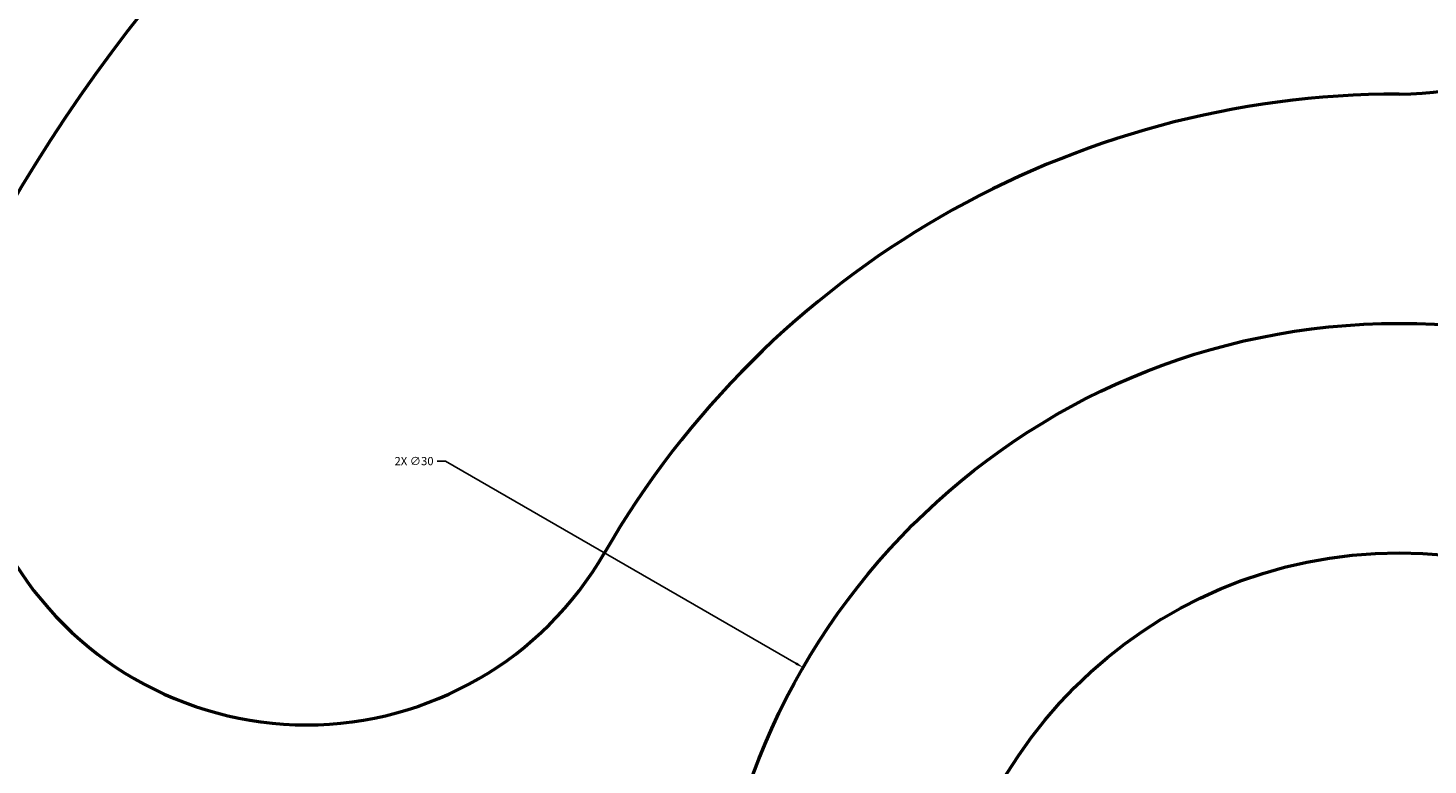
# Model space of a CAD drawing. Units: inches. Extents: x 413 to 622, y 326 to 447.
# Tile 4 of 15: x 443 to 473, y 392 to 408. Entities that reach past the tile are written whole.
import ezdxf

# ---------------------------------------------------------------- set-up
doc = ezdxf.new("R2010")
doc.units = ezdxf.units.IN
doc.header["$MEASUREMENT"] = 0
doc.layers.add('M-DIMS', color=2, linetype='Continuous', lineweight=18)
doc.layers.add('M-OUTL', color=7, linetype='Continuous', lineweight=50)
doc.styles.get("Standard").update_dxf_attribs({"font": 'arial.ttf'})
doc.dimstyles.get("Standard").update_dxf_attribs({"dimtxt": 0.18, "dimasz": 0.18, "dimexe": 0.18, "dimexo": 0.0625, "dimgap": 0.09, "dimtad": 0, "dimtih": 1, "dimtoh": 1, "dimdec": 4, "dimzin": 0, "dimdsep": 46, "dimtxsty": 'Standard', "dimcen": 0.09, "dimadec": 0, "dimazin": 0, "dimtfac": 1, "dimtdec": 4, "dimtofl": 0, "dimtmove": 0, "dimatfit": 3, "dimfxl": 1, "dimtolj": 1, "dimtzin": 0, "dimarcsym": 0})

# ---------------------------------------------------------------- blocks, each defined once
blk = doc.blocks.new('SPROCKET-HUB-BORE')
for radius in [15, 10]:
    blk.add_circle((15, 15), radius)
blk = doc.blocks.new('SPROCKET-WEB-SLOT')
for centre, radius, start, end in [((7.501, 21.25), 7.5, 30, 210), ((31.317, 35), 20, 210, 270), ((31.317, 35), 35, 210, 270), ((31.317, 7.5), 7.5, 270, 90)]:
    blk.add_arc(centre, radius, start, end)
blk = doc.blocks.new('*D10')
at = {"layer": 'Defpoints', "color": 0, "transparency": 16777216}
for p in [(413.283, 436.392), (472.684, 436.392), (472.684, 336.392)]:
    blk.add_point(p, dxfattribs=at)
at = {"layer": 'M-DIMS', "color": 0, "lineweight": -2, "transparency": 16777216}
for p, q in [((472.621, 436.392), (413.103, 436.392)), ((413.283, 436.212), (413.283, 386.573)), ((413.283, 336.572), (413.283, 386.21)), ((472.621, 336.392), (413.103, 336.392))]:
    blk.add_line(p, q, dxfattribs=at)
at = {"layer": 'M-DIMS', "color": 0, "transparency": 16777216}
for points in [[(413.253, 436.212), (413.313, 436.212), (413.283, 436.392)], [(413.253, 336.572), (413.313, 336.572), (413.283, 336.392)]]:
    blk.add_solid(points, dxfattribs=at)
at = {"layer": 'M-DIMS', "color": 0, "transparency": 16777216, "insert": (413.283, 386.392), "char_height": 0.18, "attachment_point": 5}
blk.add_mtext('\\A1;100', dxfattribs=at)
blk = doc.blocks.new('*D11')
at = {"layer": 'Defpoints', "color": 0, "transparency": 16777216}
for p in [(621.66, 446.422), (621.66, 388.074), (423.314, 378.888)]:
    blk.add_point(p, dxfattribs=at)
at = {"layer": 'M-DIMS', "color": 0, "lineweight": -2, "transparency": 16777216}
for p, q in [((423.314, 378.95), (423.314, 446.602)), ((621.66, 388.137), (621.66, 446.602)), ((423.494, 446.422), (522.031, 446.422)), ((621.48, 446.422), (522.943, 446.422))]:
    blk.add_line(p, q, dxfattribs=at)
at = {"layer": 'M-DIMS', "color": 0, "transparency": 16777216}
for points in [[(423.494, 446.452), (423.494, 446.392), (423.314, 446.422)], [(621.48, 446.452), (621.48, 446.392), (621.66, 446.422)]]:
    blk.add_solid(points, dxfattribs=at)
at = {"layer": 'M-DIMS', "color": 0, "transparency": 16777216, "insert": (522.487, 446.422), "char_height": 0.18, "attachment_point": 5}
blk.add_mtext('\\A1;198.35', dxfattribs=at)
blk = doc.blocks.new('*D13')
at = {"layer": 'Defpoints', "color": 0, "transparency": 16777216}
for p in [(413.283, 431.392), (472.684, 431.392), (472.684, 386.392)]:
    blk.add_point(p, dxfattribs=at)
at = {"layer": 'M-DIMS', "color": 0, "lineweight": -2, "transparency": 16777216}
for p, q in [((472.621, 431.392), (413.103, 431.392)), ((413.283, 431.212), (413.283, 409.073)), ((413.283, 386.572), (413.283, 408.71)), ((472.621, 386.392), (413.103, 386.392))]:
    blk.add_line(p, q, dxfattribs=at)
at = {"layer": 'M-DIMS', "color": 0, "transparency": 16777216}
for points in [[(413.253, 431.212), (413.313, 431.212), (413.283, 431.392)], [(413.253, 386.572), (413.313, 386.572), (413.283, 386.392)]]:
    blk.add_solid(points, dxfattribs=at)
at = {"layer": 'M-DIMS', "color": 0, "transparency": 16777216, "insert": (413.283, 408.892), "char_height": 0.18, "attachment_point": 5}
blk.add_mtext('\\A1;45', dxfattribs=at)
blk = doc.blocks.new('*D26')
at = {"layer": 'Defpoints', "color": 0, "transparency": 16777216}
for p in [(459.693, 393.89), (485.675, 378.893)]:
    blk.add_point(p, dxfattribs=at)
at = {"layer": 'M-DIMS', "color": 0, "lineweight": -2, "transparency": 16777216}
for p, q in [((451.718, 398.39), (451.898, 398.39)), ((451.898, 398.39), (459.537, 393.98)), ((472.594, 386.392), (472.774, 386.392)), ((472.684, 386.302), (472.684, 386.482))]:
    blk.add_line(p, q, dxfattribs=at)
at = {"layer": 'M-DIMS', "color": 0, "transparency": 16777216}
blk.add_solid([(459.552, 394.006), (459.522, 393.954), (459.693, 393.89)], dxfattribs=at)
at = {"layer": 'M-DIMS', "color": 0, "transparency": 16777216, "insert": (451.211, 398.39), "char_height": 0.18, "attachment_point": 5}
blk.add_mtext('\\A1;2X ∅30', dxfattribs=at)
blk = doc.blocks.new('*D28')
at = {"layer": 'Defpoints', "color": 0, "transparency": 16777216}
for p in [(455.184, 416.702), (472.684, 386.392)]:
    blk.add_point(p, dxfattribs=at)
at = {"layer": 'M-DIMS', "color": 0, "lineweight": -2, "transparency": 16777216}
for p, q in [((444.504, 434.889), (444.684, 434.889)), ((444.684, 434.889), (455.094, 416.858)), ((472.594, 386.392), (472.774, 386.392)), ((472.684, 386.302), (472.684, 386.482))]:
    blk.add_line(p, q, dxfattribs=at)
at = {"layer": 'M-DIMS', "color": 0, "transparency": 16777216}
blk.add_solid([(455.12, 416.873), (455.068, 416.843), (455.184, 416.702)], dxfattribs=at)
at = {"layer": 'M-DIMS', "color": 0, "transparency": 16777216, "insert": (444.005, 434.889), "char_height": 0.18, "attachment_point": 5}
blk.add_mtext('\\A1;3X R35', dxfattribs=at)

msp = doc.modelspace()

# ---------------------------------------------------------------- linework, layer by layer
at = {"layer": 'M-OUTL'}
msp.add_circle((472.6836, 386.3915), 40, dxfattribs=at)

# ---------------------------------------------------------------- block references
at = {"layer": 'M-OUTL', "rotation": 239.9999999999996}
msp.add_blockref('SPROCKET-WEB-SLOT', (458.0314, 431.0122), dxfattribs=at)
at = {"layer": 'M-OUTL'}
msp.add_blockref('SPROCKET-HUB-BORE', (457.684, 371.392), dxfattribs=at)

# ---------------------------------------------------------------- dimensions: what is measured, and where the dimension line sits
at = {"layer": 'M-DIMS'}
dim = msp.add_linear_dim(base=(621.66, 446.422), p1=(423.3136, 378.8878), p2=(621.66, 388.0741), dimstyle='Standard', override={"dimdec": 2, "dimlfac": 1, "dimrnd": 0, "dimzin": 0, "dimdsep": 46, "dimlunit": 2}, dxfattribs=at)
dim.commit()
dim.dimension.update_dxf_attribs({"geometry": '*D11', "text_midpoint": (522.4868, 446.422)})
for base, p1, p2, picture, middle in [((413.2831, 436.3915), (472.6836, 336.3915), (472.6836, 436.3915), '*D10', (413.2831, 386.3915)), ((413.2831, 431.3915), (472.6836, 386.3915), (472.6836, 431.3915), '*D13', (413.2831, 408.8915))]:
    dim = msp.add_linear_dim(base=base, p1=p1, p2=p2, angle=90, dimstyle='Standard', override={"dimdec": 0, "dimlfac": 1, "dimrnd": 0, "dimzin": 0, "dimdsep": 46, "dimlunit": 2}, dxfattribs=at)
    dim.commit()
    dim.dimension.update_dxf_attribs({"geometry": picture, "text_midpoint": middle})
dim = msp.add_radius_dim(center=(472.6836, 386.3915), mpoint=(455.1837, 416.7025), text='3X <>', dimstyle='Standard', override={"dimdec": 0, "dimlfac": 1, "dimrnd": 0, "dimzin": 0, "dimdsep": 46, "dimlunit": 2}, dxfattribs=at)
dim.commit()
dim.dimension.update_dxf_attribs({"geometry": '*D28', "text_midpoint": (444.0048, 434.889), "dimtype": 164})
dim = msp.add_diameter_dim_2p(p1=(485.6746, 378.8925), p2=(459.6926, 393.8905), text='2X <>', dimstyle='Standard', override={"dimdec": 0, "dimlfac": 1, "dimrnd": 0, "dimzin": 0, "dimdsep": 46, "dimlunit": 2}, dxfattribs=at)
dim.commit()
dim.dimension.update_dxf_attribs({"geometry": '*D26', "text_midpoint": (451.2114, 398.3899), "dimtype": 163})

doc.saveas('drawing.dxf')
